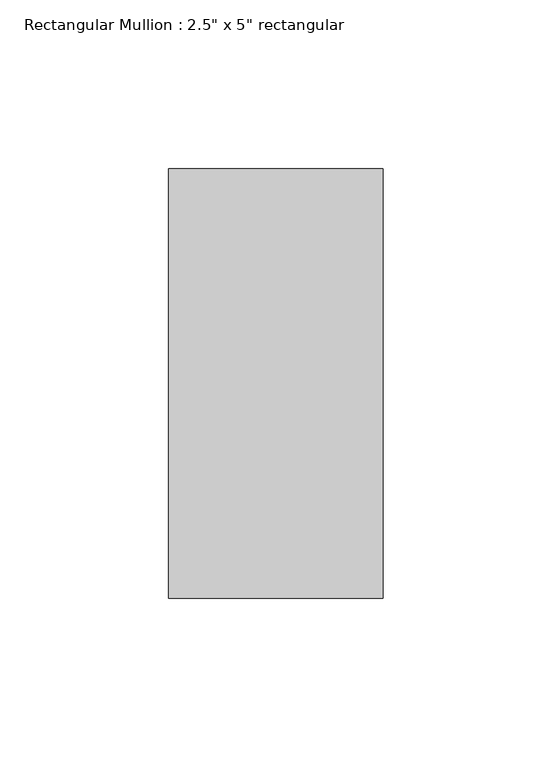
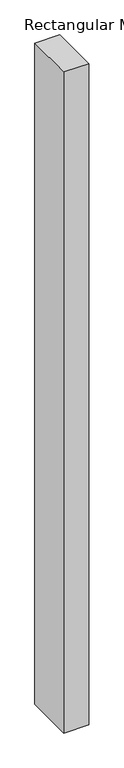
"""IFC4 building model written with IfcOpenShell, lengths in millimetres: member geometry."""

from ifc_helpers import new_model, si_unit, frame, origin, place, context, project, spatial, polyline, outline, extrude, source, transform, mapped, element, save


def member_e97ac6c9(model_context):
    return source(origin(), model_context, "Body", "SweptSolid", [
        extrude(outline(polyline([(0.0, 63.5), (0.0, -63.5), (-63.5, -63.5), (-63.5, 63.5), (0.0, 63.5)])), frame((0.0, 0.0, -1778.0), z_axis=(0.0, 0.0, 1.0), x_axis=(1.0, 0.0, 0.0)), (0.0, 0.0, 1.0), 1778.0),
    ])


if __name__ == "__main__":
    model = new_model("IFC4")
    model_context = context("Model", 3, world=origin())
    ifc_project = project(units=[si_unit("LENGTHUNIT", "METRE", prefix="MILLI")], contexts=[model_context])
    site = spatial("IfcSite", under=ifc_project)
    building = spatial("IfcBuilding", under=site)
    placement = place(None, origin())
    member_shape = member_e97ac6c9(model_context)
    element("IfcMember", 1, ObjectType="Rectangular Mullion : 2.5\" x 5\" rectangular", at=placement, inside=building, context=model_context, shape_type="MappedRepresentation", body=[
        mapped(member_shape, transform((0.0, 0.0, 0.0), x_axis=(1.0, 0.0, 0.0), y_axis=(0.0, 1.0, 0.0), z_axis=(0.0, 0.0, 1.0))),
    ])
    save(model, "model.ifc")

# Revit data of these elements
# Type "Rectangular Mullion : 2.5\" x 5\" rectangular"
#   built-in parameter 1007304 = 0.416667 (stored number, unit not read)
#   built-in parameter 1007301 = 0.104167 (stored number, unit not read)
#   built-in parameter 1007300 = 0.104167 (stored number, unit not read)
# Element 1 (IfcMember, "Rectangular Mullion : 2.5\" x 5\" rectangular")
#   Materials on its faces: "Aluminum"
# Materials
#   "Aluminum": class "Metal", colour RGB 247 247 247, transparency 0, Description = "Aluminum 6061", Cost = 0
